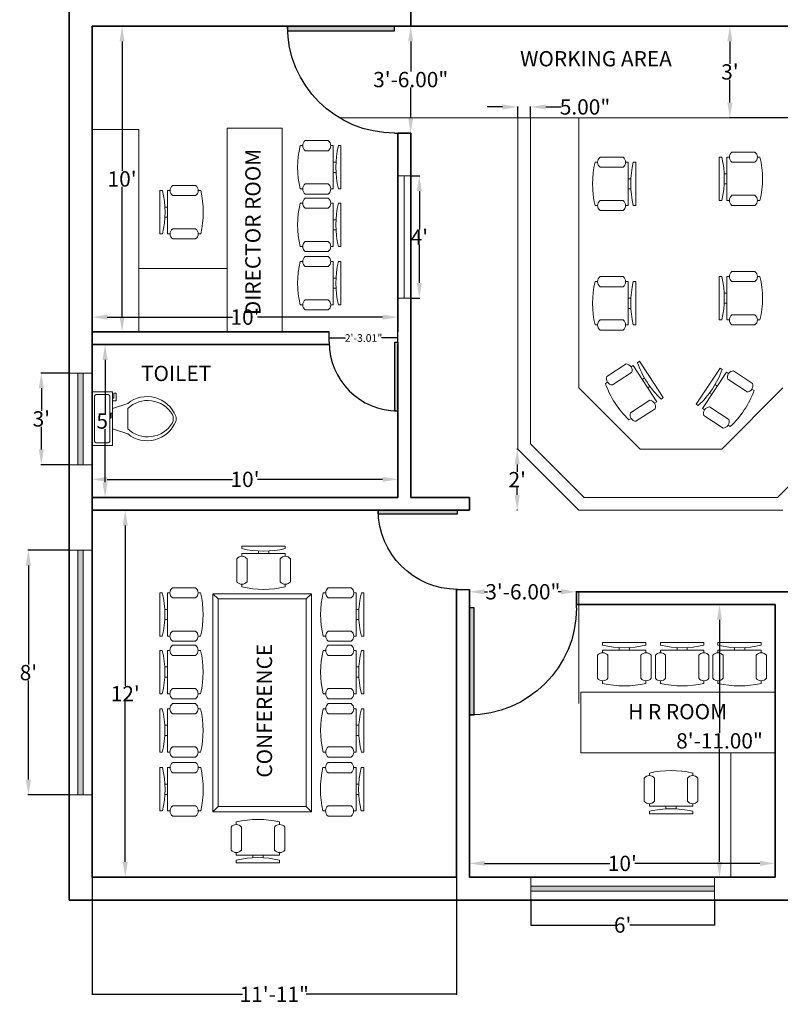
# Model space of a CAD drawing. Units: inches. Extents: x -57 to 1512, y -896 to 149.
# Tile 4 of 6: x 913 to 1211, y -647 to -261. Entities that reach past the tile are written whole.
import ezdxf

# ---------------------------------------------------------------- set-up
doc = ezdxf.new("R2010")
doc.units = ezdxf.units.IN
doc.header["$MEASUREMENT"] = 0
doc.layers.get('Defpoints').update_dxf_attribs({"color": 9})
for name, color, linetype, lineweight in [('A-ANNO-DIMS', 2, 'Continuous', 18), ('A-AREA-IDEN', 7, 'Continuous', 18), ('A-DOOR', 3, 'Continuous', 25), ('A-DOOR-PATT', 3, 'Continuous', 13), ('A-FLOR-FIXT', 9, 'Continuous', 18), ('A-FURN', 8, 'Continuous', 18), ('A-GLAZ', 4, 'Continuous', 18), ('A-GLAZ-PATT', 4, 'Continuous', 13), ('A-WALL', 7, 'Continuous', 35)]:
    doc.layers.add(name, color=color, linetype=linetype, lineweight=lineweight)
doc.styles.get("Standard").update_dxf_attribs({"font": 'arial.ttf'})
doc.dimstyles.get("Standard").update_dxf_attribs({"dimtxt": 6, "dimasz": 0.18, "dimexe": 0.18, "dimexo": 0.0625, "dimgap": 0.09, "dimtad": 0, "dimtih": 1, "dimtoh": 1, "dimzin": 0, "dimdsep": 46, "dimlunit": 3, "dimtxsty": 'Standard', "dimcen": 0.09, "dimadec": 0, "dimazin": 0, "dimtfac": 1, "dimtofl": 0, "dimtmove": 0, "dimatfit": 3, "dimfxl": 1, "dimtolj": 1, "dimtzin": 0, "dimarcsym": 0})

# ---------------------------------------------------------------- blocks, each defined once
blk = doc.blocks.new('*U2')
for p, q in [((0, 0), (0, -6)), ((40, 0), (40, -6))]:
    blk.add_line(p, q)
blk.add_lwpolyline([(0, 0), (0, 40), (1.75, 40), (1.75, 0)], close=True)
blk.add_arc((0, 0), 40, 0, 90)
blk = doc.blocks.new('*D38')
at = {"layer": 'A-ANNO-DIMS', "color": 0, "lineweight": -2, "transparency": 16777216}
for p, q in [((1066.53, -263.42), (1066.65, -263.42)), ((1066.47, -269.42), (1066.47, -281.27)), ((1066.47, -299.42), (1066.47, -287.58)), ((1066.53, -305.42), (1066.65, -305.42))]:
    blk.add_line(p, q, dxfattribs=at)
at = {"layer": 'A-ANNO-DIMS', "color": 0, "transparency": 16777216}
for points in [[(1065.47, -269.42), (1067.47, -269.42), (1066.47, -263.42)], [(1065.47, -299.42), (1067.47, -299.42), (1066.47, -305.42)]]:
    blk.add_solid(points, dxfattribs=at)
at = {"layer": 'Defpoints', "color": 0, "transparency": 16777216}
for p in [(1066.47, -263.42), (1066.47, -305.42), (1066.47, -305.42)]:
    blk.add_point(p, dxfattribs=at)
at = {"layer": 'A-ANNO-DIMS', "color": 0, "transparency": 16777216, "insert": (1066.47, -284.42), "char_height": 6, "attachment_point": 5}
blk.add_mtext('\\A1;3\'-6.00"', dxfattribs=at)
blk = doc.blocks.new('*D39')
at = {"layer": 'A-ANNO-DIMS', "color": 0, "lineweight": -2, "transparency": 16777216}
for p, q in [((1034.46, -387.41), (1034.46, -385.65)), ((1034.64, -385.83), (1040.95, -385.83)), ((1061.29, -385.83), (1054.98, -385.83)), ((1061.47, -387.41), (1061.47, -385.65))]:
    blk.add_line(p, q, dxfattribs=at)
at = {"layer": 'A-ANNO-DIMS', "color": 0, "transparency": 16777216}
for points in [[(1034.64, -385.8), (1034.64, -385.86), (1034.46, -385.83)], [(1061.29, -385.8), (1061.29, -385.86), (1061.47, -385.83)]]:
    blk.add_solid(points, dxfattribs=at)
at = {"layer": 'Defpoints', "color": 0, "transparency": 16777216}
for p in [(1034.46, -385.83), (1034.46, -387.47), (1061.47, -387.47)]:
    blk.add_point(p, dxfattribs=at)
at = {"layer": 'A-ANNO-DIMS', "color": 0, "transparency": 16777216, "insert": (1047.96, -385.83), "char_height": 3, "attachment_point": 5}
blk.add_mtext('\\A1;2\'-3.01"', dxfattribs=at)
blk = doc.blocks.new('*D40')
at = {"layer": 'A-ANNO-DIMS', "color": 0, "lineweight": -2, "transparency": 16777216}
for p, q in [((1089.47, -485.36), (1089.47, -485.24)), ((1095.47, -485.42), (1096.58, -485.42)), ((1125.47, -485.42), (1124.36, -485.42)), ((1131.47, -485.36), (1131.47, -485.24))]:
    blk.add_line(p, q, dxfattribs=at)
at = {"layer": 'A-ANNO-DIMS', "color": 0, "transparency": 16777216}
for points in [[(1095.47, -484.42), (1095.47, -486.42), (1089.47, -485.42)], [(1125.47, -484.42), (1125.47, -486.42), (1131.47, -485.42)]]:
    blk.add_solid(points, dxfattribs=at)
at = {"layer": 'Defpoints', "color": 0, "transparency": 16777216}
for p in [(1089.47, -485.42), (1089.47, -485.42), (1131.47, -485.42)]:
    blk.add_point(p, dxfattribs=at)
at = {"layer": 'A-ANNO-DIMS', "color": 0, "transparency": 16777216, "insert": (1110.47, -485.42), "char_height": 6, "attachment_point": 5}
blk.add_mtext('\\A1;3\'-6.00"', dxfattribs=at)
blk = doc.blocks.new('*D41')
at = {"layer": 'A-ANNO-DIMS', "color": 0, "lineweight": -2, "transparency": 16777216}
for p, q in [((932.41, -399.58), (921.42, -399.58)), ((921.6, -405.58), (921.6, -414.43)), ((921.6, -429.58), (921.6, -420.74)), ((932.41, -435.58), (921.42, -435.58))]:
    blk.add_line(p, q, dxfattribs=at)
at = {"layer": 'A-ANNO-DIMS', "color": 0, "transparency": 16777216}
for points in [[(920.6, -405.58), (922.6, -405.58), (921.6, -399.58)], [(920.6, -429.58), (922.6, -429.58), (921.6, -435.58)]]:
    blk.add_solid(points, dxfattribs=at)
at = {"layer": 'Defpoints', "color": 0, "transparency": 16777216}
for p in [(932.47, -399.58), (921.6, -435.58), (932.47, -435.58)]:
    blk.add_point(p, dxfattribs=at)
at = {"layer": 'A-ANNO-DIMS', "color": 0, "transparency": 16777216, "insert": (921.6, -417.58), "char_height": 6, "attachment_point": 5}
blk.add_mtext("\\A1;3'", dxfattribs=at)
blk = doc.blocks.new('*D42')
at = {"layer": 'A-ANNO-DIMS', "color": 0, "lineweight": -2, "transparency": 16777216}
for p, q in [((932.41, -469.14), (916.34, -469.14)), ((916.52, -475.14), (916.52, -513.99)), ((916.52, -559.14), (916.52, -520.3)), ((932.41, -565.14), (916.34, -565.14))]:
    blk.add_line(p, q, dxfattribs=at)
at = {"layer": 'A-ANNO-DIMS', "color": 0, "transparency": 16777216}
for points in [[(915.52, -475.14), (917.52, -475.14), (916.52, -469.14)], [(915.52, -559.14), (917.52, -559.14), (916.52, -565.14)]]:
    blk.add_solid(points, dxfattribs=at)
at = {"layer": 'Defpoints', "color": 0, "transparency": 16777216}
for p in [(932.47, -469.14), (916.52, -565.14), (932.47, -565.14)]:
    blk.add_point(p, dxfattribs=at)
at = {"layer": 'A-ANNO-DIMS', "color": 0, "transparency": 16777216, "insert": (916.52, -517.14), "char_height": 6, "attachment_point": 5}
blk.add_mtext("\\A1;8'", dxfattribs=at)
blk = doc.blocks.new('*D43')
at = {"layer": 'A-ANNO-DIMS', "color": 0, "lineweight": -2, "transparency": 16777216}
for p, q in [((1113.59, -606.48), (1113.59, -616.38)), ((1185.59, -606.48), (1185.59, -616.38)), ((1113.77, -616.2), (1146.72, -616.2)), ((1185.41, -616.2), (1152.46, -616.2))]:
    blk.add_line(p, q, dxfattribs=at)
at = {"layer": 'A-ANNO-DIMS', "color": 0, "transparency": 16777216}
for points in [[(1113.77, -616.17), (1113.77, -616.23), (1113.59, -616.2)], [(1185.41, -616.17), (1185.41, -616.23), (1185.59, -616.2)]]:
    blk.add_solid(points, dxfattribs=at)
at = {"layer": 'Defpoints', "color": 0, "transparency": 16777216}
for p in [(1113.59, -606.42), (1185.59, -606.42), (1185.59, -616.2)]:
    blk.add_point(p, dxfattribs=at)
at = {"layer": 'A-ANNO-DIMS', "color": 0, "transparency": 16777216, "insert": (1149.59, -616.2), "char_height": 6, "attachment_point": 5}
blk.add_mtext("\\A1;6'", dxfattribs=at)
blk = doc.blocks.new('Chair - Desk')
for p, q in [((-8.5, 0), (-8.5, -1)), ((-8.5, 0), (8.5, 0)), ((8.5, 0), (8.5, -1)), ((-8.5, -3), (-8.5, -4)), ((-8.5, -3), (8.5, -3)), ((-2, -3), (-2, -1.9355)), ((2, -1.9576), (2, -3)), ((8.5, -3), (8.5, -4)), ((-10.5, -5), (-10.5, -14)), ((-6.5, -14), (-6.5, -5)), ((6.5, -5), (6.5, -14)), ((10.5, -14), (10.5, -5)), ((-8.5, -15), (-8.5, -16)), ((8.5, -15), (8.5, -16))]:
    blk.add_line(p, q)
for centre, radius, start, end in [((0, 34.625), 36.625, 256.5803, 283.4197), ((-8.5, -6.5), 2.5, 36.8699, 143.1301), ((8.5, -6.5), 2.5, 36.8699, 143.1301), ((-8.5, -12.5), 2.5, 216.8699, 323.1301), ((8.5, -12.5), 2.5, 216.8699, 323.1301), ((0, 19.625), 36.625, 256.5803, 283.4197)]:
    blk.add_arc(centre, radius, start, end)
blk = doc.blocks.new('*U24')
for p, q in [((9.5, -6), (9.5, -2)), ((-10, -8.5), (-8, -8.5)), ((-10, -9.5), (-10, -8.5)), ((-7, -9.5), (-10, -9.5)), ((-8, -8.5), (-8, -8)), ((-7, -8), (-7, -9.5)), ((-4, -8), (-6, -14)), ((4, -8), (6, -14)), ((4, -14), (-4, -14))]:
    blk.add_line(p, q)
blk.add_lwpolyline([(10.5, -8), (10.5, 0), (-10.5, 0), (-10.5, -8)], close=True)
for points in [[(-9.5, -2), (-9.5, -6)], [(8.5, -1), (-8.5, -1)], [(-8.5, -7), (8.5, -7)]]:
    blk.add_lwpolyline(points)
for centre, radius, start, end in [((-8.62, -1.88), 0.884, 81.8699, 188.1301), ((8.62, -1.88), 0.884, 351.8699, 98.1301), ((-8.62, -6.12), 0.884, 171.8699, 278.1301), ((8.62, -6.12), 0.884, 261.8699, 8.1301), ((3.52, -21.58), 12.17, 141.4691, 247.9714), ((4.2, -21.82), 11.33, 136.3677, 238.9468), ((-3.52, -21.58), 12.17, 292.0284, 38.5307), ((-4.2, -21.82), 11.33, 301.053, 43.6321), ((0, -27.88), 4, 245.7318, 294.2682), ((0, -29), 4, 254.8605, 285.1395)]:
    blk.add_arc(centre, radius, start, end)
blk = doc.blocks.new('*D56')
at = {"layer": 'A-ANNO-DIMS', "color": 0, "lineweight": -2, "transparency": 16777216}
for p, q in [((1066.53, -322.21), (1070.05, -322.21)), ((1069.87, -328.21), (1069.87, -343.12)), ((1069.87, -364.21), (1069.87, -349.3)), ((1066.53, -370.21), (1070.05, -370.21))]:
    blk.add_line(p, q, dxfattribs=at)
at = {"layer": 'A-ANNO-DIMS', "color": 0, "transparency": 16777216}
for points in [[(1068.87, -328.21), (1070.87, -328.21), (1069.87, -322.21)], [(1068.87, -364.21), (1070.87, -364.21), (1069.87, -370.21)]]:
    blk.add_solid(points, dxfattribs=at)
at = {"layer": 'Defpoints', "color": 0, "transparency": 16777216}
for p in [(1066.47, -322.21), (1066.47, -370.21), (1069.87, -370.21)]:
    blk.add_point(p, dxfattribs=at)
at = {"layer": 'A-ANNO-DIMS', "color": 0, "transparency": 16777216, "insert": (1069.87, -346.21), "char_height": 6, "attachment_point": 5}
blk.add_mtext("\\A1;4'", dxfattribs=at)
blk = doc.blocks.new('*D58')
at = {"layer": 'A-ANNO-DIMS', "color": 0, "lineweight": -2, "transparency": 16777216}
for p, q in [((1214.83, -263.42), (1191.49, -263.42)), ((1191.67, -269.42), (1191.67, -278.27)), ((1191.67, -293.42), (1191.67, -284.58)), ((1214.83, -299.42), (1191.49, -299.42))]:
    blk.add_line(p, q, dxfattribs=at)
at = {"layer": 'A-ANNO-DIMS', "color": 0, "transparency": 16777216}
for points in [[(1190.67, -269.42), (1192.67, -269.42), (1191.67, -263.42)], [(1190.67, -293.42), (1192.67, -293.42), (1191.67, -299.42)]]:
    blk.add_solid(points, dxfattribs=at)
at = {"layer": 'Defpoints', "color": 0, "transparency": 16777216}
for p in [(1214.89, -263.42), (1191.67, -299.42), (1214.89, -299.42)]:
    blk.add_point(p, dxfattribs=at)
at = {"layer": 'A-ANNO-DIMS', "color": 0, "transparency": 16777216, "insert": (1191.67, -281.42), "char_height": 6, "attachment_point": 5}
blk.add_mtext("\\A1;3'", dxfattribs=at)
blk = doc.blocks.new('*D59')
at = {"layer": 'A-ANNO-DIMS', "color": 0, "lineweight": -2, "transparency": 16777216}
for p, q in [((1102.47, -295.16), (1096.47, -295.16)), ((1108.47, -299.36), (1108.47, -294.98)), ((1113.47, -299.36), (1113.47, -294.98)), ((1119.47, -295.16), (1125.47, -295.16))]:
    blk.add_line(p, q, dxfattribs=at)
at = {"layer": 'A-ANNO-DIMS', "color": 0, "transparency": 16777216}
for points in [[(1102.47, -294.16), (1102.47, -296.16), (1108.47, -295.16)], [(1119.47, -294.16), (1119.47, -296.16), (1113.47, -295.16)]]:
    blk.add_solid(points, dxfattribs=at)
at = {"layer": 'Defpoints', "color": 0, "transparency": 16777216}
for p in [(1113.47, -295.16), (1108.47, -299.42), (1113.47, -299.42)]:
    blk.add_point(p, dxfattribs=at)
at = {"layer": 'A-ANNO-DIMS', "color": 0, "transparency": 16777216, "insert": (1134.84, -295.16), "char_height": 6, "attachment_point": 5}
blk.add_mtext('\\A1;5.00"', dxfattribs=at)
blk = doc.blocks.new('*D60')
at = {"layer": 'A-ANNO-DIMS', "color": 0, "lineweight": -2, "transparency": 16777216}
for p, q in [((1108.41, -429.42), (1108.07, -429.42)), ((1108.25, -435.42), (1108.25, -438.32)), ((1108.25, -447.42), (1108.25, -444.52)), ((1108.41, -453.42), (1108.07, -453.42))]:
    blk.add_line(p, q, dxfattribs=at)
at = {"layer": 'A-ANNO-DIMS', "color": 0, "transparency": 16777216}
for points in [[(1107.25, -435.42), (1109.25, -435.42), (1108.25, -429.42)], [(1107.25, -447.42), (1109.25, -447.42), (1108.25, -453.42)]]:
    blk.add_solid(points, dxfattribs=at)
at = {"layer": 'Defpoints', "color": 0, "transparency": 16777216}
for p in [(1108.47, -429.42), (1108.25, -453.42), (1108.47, -453.42)]:
    blk.add_point(p, dxfattribs=at)
at = {"layer": 'A-ANNO-DIMS', "color": 0, "transparency": 16777216, "insert": (1108.25, -441.42), "char_height": 6, "attachment_point": 5}
blk.add_mtext("\\A1;2'", dxfattribs=at)
blk = doc.blocks.new('*D72')
at = {"layer": 'A-ANNO-DIMS', "color": 0, "lineweight": -2, "transparency": 16777216}
for p, q in [((1089.47, -597.36), (1089.47, -591.82)), ((1095.47, -592), (1144.57, -592)), ((1203.47, -592), (1154.37, -592)), ((1209.47, -597.36), (1209.47, -591.82))]:
    blk.add_line(p, q, dxfattribs=at)
at = {"layer": 'A-ANNO-DIMS', "color": 0, "transparency": 16777216}
for points in [[(1095.47, -591), (1095.47, -593), (1089.47, -592)], [(1203.47, -591), (1203.47, -593), (1209.47, -592)]]:
    blk.add_solid(points, dxfattribs=at)
at = {"layer": 'Defpoints', "color": 0, "transparency": 16777216}
for p in [(1209.47, -592), (1089.47, -597.42), (1209.47, -597.42)]:
    blk.add_point(p, dxfattribs=at)
at = {"layer": 'A-ANNO-DIMS', "color": 0, "transparency": 16777216, "insert": (1149.47, -592), "char_height": 6, "attachment_point": 5}
blk.add_mtext("\\A1;10'", dxfattribs=at)
blk = doc.blocks.new('*D73')
at = {"layer": 'A-ANNO-DIMS', "color": 0, "lineweight": -2, "transparency": 16777216}
for p, q in [((1209.41, -490.42), (1187.41, -490.42)), ((1187.59, -496.42), (1187.59, -540.77)), ((1187.59, -591.42), (1187.59, -547.07)), ((1209.41, -597.42), (1187.41, -597.42))]:
    blk.add_line(p, q, dxfattribs=at)
at = {"layer": 'A-ANNO-DIMS', "color": 0, "transparency": 16777216}
for points in [[(1186.59, -496.42), (1188.59, -496.42), (1187.59, -490.42)], [(1186.59, -591.42), (1188.59, -591.42), (1187.59, -597.42)]]:
    blk.add_solid(points, dxfattribs=at)
at = {"layer": 'Defpoints', "color": 0, "transparency": 16777216}
for p in [(1187.59, -490.42), (1209.47, -490.42), (1209.47, -597.42)]:
    blk.add_point(p, dxfattribs=at)
at = {"layer": 'A-ANNO-DIMS', "color": 0, "transparency": 16777216, "insert": (1187.59, -543.92), "char_height": 6, "attachment_point": 5}
blk.add_mtext('\\A1;8\'-11.00"', dxfattribs=at)
blk = doc.blocks.new('*D74')
at = {"layer": 'A-ANNO-DIMS', "color": 0, "lineweight": -2, "transparency": 16777216}
for p, q in [((941.53, -453.42), (954.69, -453.42)), ((954.51, -459.42), (954.51, -522.32)), ((954.51, -591.42), (954.51, -528.52)), ((941.53, -597.42), (954.69, -597.42))]:
    blk.add_line(p, q, dxfattribs=at)
at = {"layer": 'A-ANNO-DIMS', "color": 0, "transparency": 16777216}
for points in [[(953.51, -459.42), (955.51, -459.42), (954.51, -453.42)], [(953.51, -591.42), (955.51, -591.42), (954.51, -597.42)]]:
    blk.add_solid(points, dxfattribs=at)
at = {"layer": 'Defpoints', "color": 0, "transparency": 16777216}
for p in [(941.47, -453.42), (941.47, -597.42), (954.51, -597.42)]:
    blk.add_point(p, dxfattribs=at)
at = {"layer": 'A-ANNO-DIMS', "color": 0, "transparency": 16777216, "insert": (954.51, -525.42), "char_height": 6, "attachment_point": 5}
blk.add_mtext("\\A1;12'", dxfattribs=at)
blk = doc.blocks.new('*D75')
at = {"layer": 'A-ANNO-DIMS', "color": 0, "lineweight": -2, "transparency": 16777216}
for p, q in [((941.47, -448.36), (941.47, -441.13)), ((947.47, -441.31), (996.57, -441.31)), ((1055.47, -441.31), (1006.37, -441.31)), ((1061.47, -448.36), (1061.47, -441.13))]:
    blk.add_line(p, q, dxfattribs=at)
at = {"layer": 'A-ANNO-DIMS', "color": 0, "transparency": 16777216}
for points in [[(947.47, -440.31), (947.47, -442.31), (941.47, -441.31)], [(1055.47, -440.31), (1055.47, -442.31), (1061.47, -441.31)]]:
    blk.add_solid(points, dxfattribs=at)
at = {"layer": 'Defpoints', "color": 0, "transparency": 16777216}
for p in [(1061.47, -441.31), (941.47, -448.42), (1061.47, -448.42)]:
    blk.add_point(p, dxfattribs=at)
at = {"layer": 'A-ANNO-DIMS', "color": 0, "transparency": 16777216, "insert": (1001.47, -441.31), "char_height": 6, "attachment_point": 5}
blk.add_mtext("\\A1;10'", dxfattribs=at)
blk = doc.blocks.new('*D76')
at = {"layer": 'A-ANNO-DIMS', "color": 0, "lineweight": -2, "transparency": 16777216}
for p, q in [((941.53, -388.42), (946.78, -388.42)), ((946.6, -394.42), (946.6, -415.28)), ((946.6, -442.42), (946.6, -421.56)), ((941.53, -448.42), (946.78, -448.42))]:
    blk.add_line(p, q, dxfattribs=at)
at = {"layer": 'A-ANNO-DIMS', "color": 0, "transparency": 16777216}
for points in [[(945.6, -394.42), (947.6, -394.42), (946.6, -388.42)], [(945.6, -442.42), (947.6, -442.42), (946.6, -448.42)]]:
    blk.add_solid(points, dxfattribs=at)
at = {"layer": 'Defpoints', "color": 0, "transparency": 16777216}
for p in [(941.47, -388.42), (941.47, -448.42), (946.6, -448.42)]:
    blk.add_point(p, dxfattribs=at)
at = {"layer": 'A-ANNO-DIMS', "color": 0, "transparency": 16777216, "insert": (946.6, -418.42), "char_height": 6, "attachment_point": 5}
blk.add_mtext("\\A1;5'", dxfattribs=at)
blk = doc.blocks.new('*D77')
at = {"layer": 'A-ANNO-DIMS', "color": 0, "lineweight": -2, "transparency": 16777216}
for p, q in [((941.47, -383.36), (941.47, -377.46)), ((947.47, -377.64), (996.57, -377.64)), ((1055.47, -377.64), (1006.37, -377.64)), ((1061.47, -383.36), (1061.47, -377.46))]:
    blk.add_line(p, q, dxfattribs=at)
at = {"layer": 'A-ANNO-DIMS', "color": 0, "transparency": 16777216}
for points in [[(947.47, -376.64), (947.47, -378.64), (941.47, -377.64)], [(1055.47, -376.64), (1055.47, -378.64), (1061.47, -377.64)]]:
    blk.add_solid(points, dxfattribs=at)
at = {"layer": 'Defpoints', "color": 0, "transparency": 16777216}
for p in [(1061.47, -377.64), (941.47, -383.42), (1061.47, -383.42)]:
    blk.add_point(p, dxfattribs=at)
at = {"layer": 'A-ANNO-DIMS', "color": 0, "transparency": 16777216, "insert": (1001.47, -377.64), "char_height": 6, "attachment_point": 5}
blk.add_mtext("\\A1;10'", dxfattribs=at)
blk = doc.blocks.new('*D78')
at = {"layer": 'A-ANNO-DIMS', "color": 0, "lineweight": -2, "transparency": 16777216}
for p, q in [((941.53, -263.42), (953.45, -263.42)), ((953.27, -269.42), (953.27, -320.27)), ((953.27, -377.42), (953.27, -326.57)), ((941.53, -383.42), (953.45, -383.42))]:
    blk.add_line(p, q, dxfattribs=at)
at = {"layer": 'A-ANNO-DIMS', "color": 0, "transparency": 16777216}
for points in [[(952.27, -269.42), (954.27, -269.42), (953.27, -263.42)], [(952.27, -377.42), (954.27, -377.42), (953.27, -383.42)]]:
    blk.add_solid(points, dxfattribs=at)
at = {"layer": 'Defpoints', "color": 0, "transparency": 16777216}
for p in [(941.47, -263.42), (953.27, -263.42), (941.47, -383.42)]:
    blk.add_point(p, dxfattribs=at)
at = {"layer": 'A-ANNO-DIMS', "color": 0, "transparency": 16777216, "insert": (953.27, -323.42), "char_height": 6, "attachment_point": 5}
blk.add_mtext("\\A1;10'", dxfattribs=at)
blk = doc.blocks.new('*D107')
at = {"layer": 'A-ANNO-DIMS', "color": 0, "lineweight": -2, "transparency": 16777216}
for p, q in [((941.47, -597.48), (941.47, -643.55)), ((1084.47, -597.48), (1084.47, -643.55)), ((941.65, -643.37), (1000.53, -643.37)), ((1084.29, -643.37), (1025.42, -643.37))]:
    blk.add_line(p, q, dxfattribs=at)
at = {"layer": 'A-ANNO-DIMS', "color": 0, "transparency": 16777216}
for points in [[(941.65, -643.34), (941.65, -643.4), (941.47, -643.37)], [(1084.29, -643.34), (1084.29, -643.4), (1084.47, -643.37)]]:
    blk.add_solid(points, dxfattribs=at)
at = {"layer": 'Defpoints', "color": 0, "transparency": 16777216}
for p in [(941.47, -597.42), (1084.47, -597.42), (1084.47, -643.37)]:
    blk.add_point(p, dxfattribs=at)
at = {"layer": 'A-ANNO-DIMS', "color": 0, "transparency": 16777216, "insert": (1012.97, -643.37), "char_height": 6, "attachment_point": 5}
blk.add_mtext('\\A1;11\'-11"', dxfattribs=at)

msp = doc.modelspace()

# ---------------------------------------------------------------- hatches: boundary and pattern name
at = {"layer": 'A-DOOR-PATT'}
h = msp.add_hatch(color=256, dxfattribs=at)
h.dxf.hatch_style = 1
h.paths.add_polyline_path([(1084.811, -453.421), (1053.741, -453.421, 0.0109414), (1053.771, -454.781), (1084.811, -454.781)])
h.paths.add_polyline_path([(1091.31, -491.725), (1089.471, -491.725), (1089.471, -533.753), (1091.31, -533.753)])
h.paths.add_polyline_path([(1216.31, -514.725), (1214.471, -514.725), (1214.471, -556.753, 0.0109414), (1216.31, -556.713)])
h.paths.add_polyline_path([(1312.941, -507.109), (1282.971, -507.109), (1282.971, -508.421), (1312.969, -508.421, 0.0109414)])
h.paths.add_polyline_path([(1312.941, -442.147), (1282.971, -442.147), (1282.971, -443.421), (1312.969, -443.421, 0.0106229)])
h.paths.add_polyline_path([(1302.763, -246.583), (1260.775, -246.583), (1260.775, -248.421), (1302.803, -248.421, 0.0109414)])
h.paths.add_polyline_path([(1312.941, -312.109), (1282.971, -312.109), (1282.971, -313.421), (1312.969, -313.421, 0.0109414)])
h.paths.add_polyline_path([(1312.941, -377.109), (1282.971, -377.109), (1282.971, -378.421), (1312.969, -378.421, 0.0109414)])
h.paths.add_polyline_path([(1061.471, -387.473), (1060.289, -387.473), (1060.289, -414.461, 0.0109414), (1061.471, -414.487)])
h.paths.add_polyline_path([(1060.167, -263.421), (1018.139, -263.421, 0.0109414), (1018.179, -265.26), (1060.167, -265.26)])
h.paths.add_polyline_path([(1326.803, -121.583), (1284.775, -121.583), (1284.775, -123.421), (1326.803, -123.421)])
h.paths.add_polyline_path([(980.763, -121.583), (938.775, -121.583), (938.775, -123.421), (980.803, -123.421, 0.0109414)])
h.paths.add_polyline_path([(1177.375, -188.23), (1115.807, -188.23), (1115.807, -219.221), (1177.375, -219.221)])
at = {"layer": 'A-GLAZ-PATT'}
h = msp.add_hatch(color=256, dxfattribs=at)
h.dxf.hatch_style = 1
h.paths.add_polyline_path([(1408.971, -264.791), (1406.971, -264.791), (1406.971, -300.791), (1408.971, -300.791)])
h.paths.add_polyline_path([(1384.971, -330.143), (1382.971, -330.143), (1382.971, -366.143), (1384.971, -366.143)])
h.paths.add_polyline_path([(1384.971, -460.981), (1382.971, -460.981), (1382.971, -496.981), (1384.971, -496.981)])
h.paths.add_polyline_path([(1384.971, -389.802), (1382.971, -389.802), (1382.971, -425.802), (1384.971, -425.802)])
h.paths.add_polyline_path([(937.971, -469.144), (935.971, -469.144), (935.971, -565.144), (937.971, -565.144)])
h.paths.add_polyline_path([(937.971, -399.584), (935.971, -399.584), (935.971, -435.584), (937.971, -435.584)])
h = msp.add_hatch(color=256, dxfattribs=at)
h.dxf.hatch_style = 1
h.paths.add_polyline_path([(1185.59, -600.921), (1113.59, -600.921), (1113.59, -602.921), (1185.59, -602.921)])

# ---------------------------------------------------------------- linework, layer by layer
at = {"layer": 'A-FURN'}
for p, q in [((1038.48, -299.421), (1278.471, -299.421)), ((1108.471, -299.421), (1108.471, -429.421)), ((1113.471, -299.421), (1113.471, -427.35)), ((1132.471, -299.421), (1132.471, -405.421)), ((1156.471, -429.421), (1132.471, -405.421)), ((1188.471, -429.421), (1212.471, -405.421)), ((1134.542, -448.421), (1113.471, -427.35)), ((1210.4, -448.421), (1231.471, -427.35)), ((1132.471, -453.421), (1108.471, -429.421)), ((1108.471, -429.421), (1108.471, -429.421)), ((1156.471, -429.421), (1188.471, -429.421)), ((1134.542, -448.421), (1210.4, -448.421)), ((1132.471, -453.421), (1212.471, -453.421)), ((988.924, -486.199), (990.924, -488.199)), ((1027.499, -486.199), (1025.499, -488.199)), ((1132.471, -485.421), (1132.471, -529.213)), ((990.924, -569.737), (988.924, -571.737)), ((1025.499, -569.737), (1027.499, -571.737))]:
    msp.add_line(p, q, dxfattribs=at)
for points in [[(941.471, -304.067), (959.879, -304.067), (959.879, -383.421), (941.471, -383.421)], [(994.444, -383.421), (1016.099, -383.421), (1016.099, -303.443), (994.444, -303.443)], [(941.471, -314.011), (941.471, -314.011), (941.471, -383.421), (941.471, -383.421)], [(959.879, -383.421), (994.444, -383.421), (994.444, -358.58), (959.879, -358.58)], [(988.924, -486.199), (1027.499, -486.199), (1027.499, -571.737), (988.924, -571.737)], [(990.924, -488.199), (1025.499, -488.199), (1025.499, -569.737), (990.924, -569.737)], [(1209.471, -548.607), (1133.159, -548.607), (1133.159, -524.762), (1209.471, -524.762)], [(1209.471, -597.421), (1192.038, -597.421), (1192.038, -548.607), (1209.471, -548.607)]]:
    msp.add_lwpolyline(points, close=True, dxfattribs=at)
at = {"layer": 'A-GLAZ'}
for p, q in [((1061.471, -322.214), (1066.471, -322.214)), ((1063.929, -322.214), (1063.929, -370.214)), ((1061.471, -370.214), (1066.471, -370.214)), ((941.471, -399.584), (932.471, -399.584)), ((935.971, -399.584), (935.971, -435.584)), ((937.971, -399.584), (937.971, -435.584)), ((941.471, -435.584), (932.471, -435.584)), ((941.471, -469.144), (932.471, -469.144)), ((935.971, -469.144), (935.971, -565.144)), ((937.971, -469.144), (937.971, -565.144)), ((941.471, -565.144), (932.471, -565.144)), ((1113.59, -597.421), (1113.59, -606.421)), ((1185.59, -597.421), (1185.59, -606.421)), ((1113.59, -600.921), (1185.59, -600.921)), ((1113.59, -602.921), (1185.59, -602.921))]:
    msp.add_line(p, q, dxfattribs=at)
at = {"layer": 'A-WALL'}
for p, q in [((932.471, -51.421), (932.471, -606.421)), ((1066.471, -123.421), (1066.471, -263.421)), ((941.471, -263.421), (1214.89, -263.421)), ((941.471, -263.421), (941.471, -485.421)), ((1061.471, -305.421), (1061.471, -383.421)), ((1061.471, -305.421), (1066.471, -305.421)), ((1066.471, -305.421), (1066.471, -448.421)), ((941.471, -383.421), (1034.458, -383.421)), ((941.471, -388.421), (1034.475, -388.421)), ((1061.471, -388.421), (1061.471, -448.421)), ((941.471, -448.421), (1061.471, -448.421)), ((1066.471, -448.421), (1089.471, -448.421)), ((1089.471, -448.421), (1089.471, -453.421)), ((941.471, -453.421), (941.471, -597.421)), ((941.471, -453.421), (1089.471, -453.421)), ((1084.471, -484.489), (1084.471, -597.421)), ((1089.471, -484.491), (1089.471, -597.421)), ((1131.471, -485.421), (1131.471, -490.421)), ((1131.471, -485.421), (1214.471, -485.421)), ((1131.471, -490.421), (1209.471, -490.421)), ((1209.471, -490.421), (1209.471, -597.421)), ((941.471, -597.421), (1084.471, -597.421)), ((1089.471, -597.421), (1209.471, -597.421)), ((932.471, -606.421), (1412.471, -606.421))]:
    msp.add_line(p, q, dxfattribs=at)

# ---------------------------------------------------------------- block references
at = {"layer": 'A-DOOR'}
for p, xscale, yscale, zscale, rotation in [((1060.167, -263.421), -1.050697738247698, 1.050697738247698, 1.050697738247698, 90), ((1061.471, -387.473), 0.6753329200725322, 0.6753329200725322, 0.6753329200725322, 180), ((1084.811, -453.421), -0.7767467920305179, 0.7767467920305179, 0.7767467920305179, 90), ((1089.471, -491.725), -1.050697738247698, 1.050697738247698, 1.050697738247698, 180)]:
    msp.add_blockref('*U2', p, dxfattribs=dict(at, xscale=xscale, yscale=yscale, zscale=zscale, rotation=rotation))
at = {"layer": 'A-FLOR-FIXT', "xscale": -1, "rotation": 89.9999999999968}
msp.add_blockref('*U24', (941.471, -417.497), dxfattribs=at)
at = {"layer": 'A-FURN', "xscale": -1}
for p, rotation in [((1039.119, -318.847), 270), ((1154.784, -325.347), 270), ((1039.119, -341.43), 270), ((1039.119, -364.34), 270), ((1154.784, -372.223), 270), ((1048.124, -494.332), 270), ((1048.124, -516.915), 270), ((1048.124, -539.825), 270), ((1048.06, -562.921), 270), ((1006.548, -591.758), 180)]:
    msp.add_blockref('Chair - Desk', p, dxfattribs=dict(at, rotation=rotation))
at = {"layer": 'A-FURN'}
for p, rotation in [((1187.474, -323.347), 90.00000000000003), ((968.116, -336.466), 90), ((1187.474, -370.223), 90.00000000000003), ((1160.87, -402.102), 302.9666763656253), ((1183.128, -404.701), 56.49295881673056), ((968.052, -494.332), 90), ((968.052, -516.915), 90), ((968.052, -539.825), 90), ((968.116, -562.921), 90), ((1168.573, -572.576), 180)]:
    msp.add_blockref('Chair - Desk', p, dxfattribs=dict(at, rotation=rotation))
for p in [(1008.767, -467.463), (1150.243, -505.36), (1172.943, -505.36), (1195.463, -505.36)]:
    msp.add_blockref('Chair - Desk', p, dxfattribs=at)

# ---------------------------------------------------------------- texts
at = {"layer": 'A-AREA-IDEN', "char_height": 6, "attachment_point": 1}
for s, insert in [('WORKING AREA', (1109.382, -273.244)), ('TOILET', (960.69, -396.736)), ('H R ROOM', (1151.748, -529.458))]:
    msp.add_mtext_dynamic_manual_height_columns(s, width=160.11736, gutter_width=1, heights=[0], dxfattribs=dict(at, insert=insert))
at = {"layer": 'A-AREA-IDEN', "char_height": 6, "attachment_point": 1, "rotation": 90}
for s, insert in [('DIRECTOR ROOM', (1001.576, -376.856)), ('CONFERENCE', (1006.102, -558.378))]:
    msp.add_mtext_dynamic_manual_height_columns(s, width=160.11736, gutter_width=1, heights=[0], dxfattribs=dict(at, insert=insert))

# ---------------------------------------------------------------- dimensions: what is measured, and where the dimension line sits
at = {"layer": 'A-ANNO-DIMS'}
for base, p1, p2, picture, middle in [((953.273, -263.421), (941.471, -383.421), (941.471, -263.421), '*D78', (953.273, -323.421)), ((1066.471, -305.421), (1066.471, -263.421), (1066.471, -305.421), '*D38', (1066.471, -284.421)), ((1191.669, -299.421), (1214.89, -263.421), (1214.89, -299.421), '*D58', (1191.669, -281.421)), ((1069.873, -370.214), (1066.471, -322.214), (1066.471, -370.214), '*D56', (1069.873, -346.214)), ((946.602, -448.421), (941.471, -388.421), (941.471, -448.421), '*D76', (946.602, -418.421)), ((921.603, -435.584), (932.471, -399.584), (932.471, -435.584), '*D41', (921.603, -417.584)), ((1108.247, -453.421), (1108.471, -429.421), (1108.471, -453.421), '*D60', (1108.247, -441.421)), ((954.507, -597.421), (941.471, -453.421), (941.471, -597.421), '*D74', (954.507, -525.421)), ((916.522, -565.144), (932.471, -469.144), (932.471, -565.144), '*D42', (916.522, -517.144)), ((1187.591, -490.421), (1209.471, -597.421), (1209.471, -490.421), '*D73', (1187.591, -543.921))]:
    dim = msp.add_linear_dim(base=base, p1=p1, p2=p2, angle=90, dimstyle='Standard', override={"dimasz": 6, "dimclrd": 0, "dimclre": 0, "dimclrt": 0}, dxfattribs=at)
    dim.commit()
    dim.dimension.update_dxf_attribs({"geometry": picture, "text_midpoint": middle})
for base, p1, p2, override, picture, middle in [((1113.471, -295.163), (1108.471, -299.421), (1113.471, -299.421), {"dimasz": 6, "dimclrd": 0, "dimclre": 0, "dimclrt": 0}, '*D59', (1134.835, -295.163)), ((1061.471, -377.644), (941.471, -383.421), (1061.471, -383.421), {"dimasz": 6, "dimclrd": 0, "dimclre": 0, "dimclrt": 0}, '*D77', (1001.471, -377.644)), ((1034.458, -385.834), (1061.471, -387.473), (1034.458, -387.473), {"dimtxt": 3, "dimclrd": 0, "dimclre": 0, "dimclrt": 0}, '*D39', (1047.965, -385.834)), ((1061.471, -441.314), (941.471, -448.421), (1061.471, -448.421), {"dimasz": 6, "dimclrd": 0, "dimclre": 0, "dimclrt": 0}, '*D75', (1001.471, -441.314)), ((1089.471, -485.421), (1131.471, -485.421), (1089.471, -485.421), {"dimasz": 6, "dimclrd": 0, "dimclre": 0, "dimclrt": 0}, '*D40', (1110.471, -485.421)), ((1209.471, -592.003), (1089.471, -597.421), (1209.471, -597.421), {"dimasz": 6, "dimclrd": 0, "dimclre": 0, "dimclrt": 0}, '*D72', (1149.471, -592.003)), ((1084.471, -643.371), (941.471, -597.421), (1084.471, -597.421), {"dimdec": 1, "dimlfac": 1, "dimrnd": 0, "dimzin": 1, "dimdsep": 46, "dimlunit": 4, "dimfrac": 2}, '*D107', (1012.971, -643.371)), ((1185.59, -616.2), (1113.59, -606.421), (1185.59, -606.421), {"dimclrd": 0, "dimclre": 0, "dimclrt": 0}, '*D43', (1149.59, -616.2))]:
    dim = msp.add_linear_dim(base=base, p1=p1, p2=p2, dimstyle='Standard', override=override, dxfattribs=at)
    dim.commit()
    dim.dimension.update_dxf_attribs({"geometry": picture, "text_midpoint": middle})

doc.saveas('drawing.dxf')
